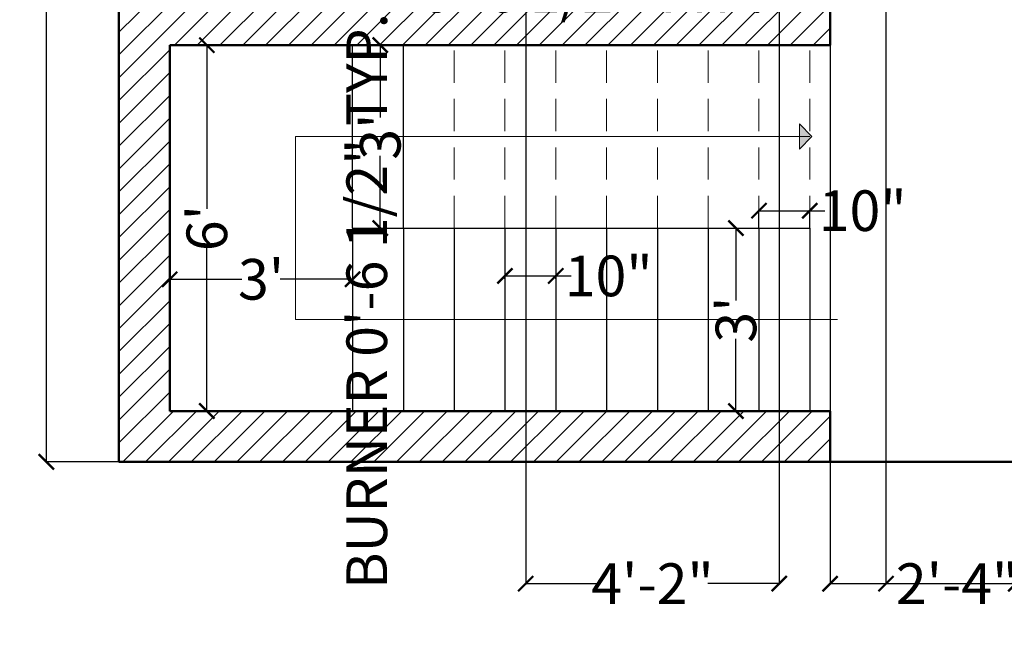
# Model space of a CAD drawing. Units: inches. Extents: x 1945 to 2401, y 1770 to 2289.
# Tile 1 of 5: x 1983 to 2177, y 1770 to 1893. Entities that reach past the tile are written whole.
import ezdxf

# ---------------------------------------------------------------- set-up
doc = ezdxf.new("R2010")
doc.units = ezdxf.units.IN
doc.linetypes.add('HIDDEN', pattern=[9.525, 6.35, -3.175])
for name, color, linetype, lineweight in [('A-ANNO-DIMS', 2, 'Continuous', 18), ('A-ANNO-SYMB', 50, 'Continuous', 18), ('A-FLOR-STRS-HIDN', 50, 'HIDDEN', 18), ('A-WALL-PATT', 8, 'Continuous', 13), ('Stairs', 50, 'Continuous', 25), ('Walls', 7, 'Continuous', 50)]:
    doc.layers.add(name, color=color, linetype=linetype, lineweight=lineweight)
doc.styles.get("Standard").update_dxf_attribs({"font": 'arial.ttf'})
doc.dimstyles.get("Standard").update_dxf_attribs({"dimtxt": 8, "dimasz": 3, "dimexe": 0.18, "dimexo": 0.0625, "dimgap": 0.09, "dimtad": 0, "dimdec": 1, "dimzin": 0, "dimdsep": 46, "dimlunit": 4, "dimtxsty": 'Standard', "dimblk": 'ARCHTICK', "dimcen": 0.09, "dimadec": 0, "dimazin": 0, "dimtfac": 1, "dimtdec": 1, "dimtofl": 0, "dimtmove": 0, "dimatfit": 3, "dimfxl": 1, "dimtolj": 1, "dimtzin": 0, "dimarcsym": 0})

# ---------------------------------------------------------------- blocks, each defined once
blk = doc.blocks.new('_ArchTick')
at = {"color": 0, "linetype": 'ByBlock', "const_width": 0.15}
blk.add_lwpolyline([(-0.5, -0.5), (0.5, 0.5)], dxfattribs=at)
blk = doc.blocks.new('*D13')
at = {"layer": 'A-ANNO-DIMS', "color": 0, "lineweight": -2, "transparency": 16777216}
for p, q in [((2123.03, 1852.04), (2124.49, 1852.04)), ((2124.31, 1852.04), (2124.31, 1837.81)), ((2124.31, 1816.04), (2124.31, 1830.27)), ((2123.03, 1816.04), (2124.49, 1816.04))]:
    blk.add_line(p, q, dxfattribs=at)
at = {"layer": 'Defpoints', "color": 0, "transparency": 16777216}
for p in [(2122.96, 1852.04), (2124.31, 1852.04), (2122.96, 1816.04)]:
    blk.add_point(p, dxfattribs=at)
at = {"layer": 'A-ANNO-DIMS', "color": 0, "lineweight": -2, "transparency": 16777216, "xscale": 3, "yscale": 3, "zscale": 3}
for p, rotation in [((2124.31, 1852.04), 90), ((2124.31, 1816.04), 270)]:
    blk.add_blockref('_ArchTick', p, dxfattribs=dict(at, rotation=rotation))
at = {"layer": 'A-ANNO-DIMS', "color": 0, "transparency": 16777216, "insert": (2124.31, 1834.04), "char_height": 8, "attachment_point": 5, "rotation": 90}
blk.add_mtext("\\A1;3'", dxfattribs=at)
blk = doc.blocks.new('*D14')
at = {"layer": 'A-ANNO-DIMS', "color": 0, "lineweight": -2, "transparency": 16777216}
for p, q in [((2048.9, 1888.04), (2054.47, 1888.04)), ((2054.29, 1888.04), (2054.29, 1873.81)), ((2054.29, 1852.04), (2054.29, 1866.27)), ((2048.9, 1852.04), (2054.47, 1852.04))]:
    blk.add_line(p, q, dxfattribs=at)
at = {"layer": 'Defpoints', "color": 0, "transparency": 16777216}
for p in [(2048.84, 1888.04), (2048.84, 1852.04), (2054.29, 1852.04)]:
    blk.add_point(p, dxfattribs=at)
at = {"layer": 'A-ANNO-DIMS', "color": 0, "lineweight": -2, "transparency": 16777216, "xscale": 3, "yscale": 3, "zscale": 3}
for p, rotation in [((2054.29, 1888.04), 90), ((2054.29, 1852.04), 270)]:
    blk.add_blockref('_ArchTick', p, dxfattribs=dict(at, rotation=rotation))
at = {"layer": 'A-ANNO-DIMS', "color": 0, "transparency": 16777216, "insert": (2054.29, 1870.04), "char_height": 8, "attachment_point": 5, "rotation": 90}
blk.add_mtext("\\A1;3'", dxfattribs=at)
blk = doc.blocks.new('*D15')
at = {"layer": 'A-ANNO-DIMS', "color": 0, "lineweight": -2, "transparency": 16777216}
for p, q in [((2012.9, 1888.04), (2020.33, 1888.04)), ((2020.15, 1888.04), (2020.15, 1855.83)), ((2020.15, 1816.04), (2020.15, 1848.25)), ((2012.9, 1816.04), (2020.33, 1816.04))]:
    blk.add_line(p, q, dxfattribs=at)
at = {"layer": 'Defpoints', "color": 0, "transparency": 16777216}
for p in [(2012.84, 1888.04), (2020.15, 1888.04), (2012.84, 1816.04)]:
    blk.add_point(p, dxfattribs=at)
at = {"layer": 'A-ANNO-DIMS', "color": 0, "lineweight": -2, "transparency": 16777216, "xscale": 3, "yscale": 3, "zscale": 3}
for p, rotation in [((2020.15, 1888.04), 90), ((2020.15, 1816.04), 270)]:
    blk.add_blockref('_ArchTick', p, dxfattribs=dict(at, rotation=rotation))
at = {"layer": 'A-ANNO-DIMS', "color": 0, "transparency": 16777216, "insert": (2020.15, 1852.04), "char_height": 8, "attachment_point": 5, "rotation": 90}
blk.add_mtext("\\A1;6'", dxfattribs=at)
blk = doc.blocks.new('*D16')
at = {"layer": 'A-ANNO-DIMS', "color": 0, "lineweight": -2, "transparency": 16777216}
for p, q in [((2012.84, 1851.98), (2012.84, 1841.78)), ((2048.84, 1851.98), (2048.84, 1841.78)), ((2012.84, 1841.96), (2027.07, 1841.96)), ((2048.84, 1841.96), (2034.61, 1841.96))]:
    blk.add_line(p, q, dxfattribs=at)
at = {"layer": 'Defpoints', "color": 0, "transparency": 16777216}
for p in [(2012.84, 1852.04), (2048.84, 1852.04), (2012.84, 1841.96)]:
    blk.add_point(p, dxfattribs=at)
at = {"layer": 'A-ANNO-DIMS', "color": 0, "lineweight": -2, "transparency": 16777216, "xscale": 3, "yscale": 3, "zscale": 3, "rotation": 180}
blk.add_blockref('_ArchTick', (2012.84, 1841.96), dxfattribs=at)
at = {"layer": 'A-ANNO-DIMS', "color": 0, "lineweight": -2, "transparency": 16777216, "xscale": 3, "yscale": 3, "zscale": 3}
blk.add_blockref('_ArchTick', (2048.84, 1841.96), dxfattribs=at)
at = {"layer": 'A-ANNO-DIMS', "color": 0, "transparency": 16777216, "insert": (2030.84, 1841.96), "char_height": 8, "attachment_point": 5}
blk.add_mtext("\\A1;3'", dxfattribs=at)
blk = doc.blocks.new('*D17')
at = {"layer": 'A-ANNO-DIMS', "color": 0, "lineweight": -2, "transparency": 16777216}
for p, q in [((2078.84, 1842.02), (2078.84, 1842.8)), ((2078.84, 1842.62), (2088.84, 1842.62)), ((2088.84, 1842.02), (2088.84, 1842.8)), ((2088.84, 1842.62), (2091.84, 1842.62))]:
    blk.add_line(p, q, dxfattribs=at)
at = {"layer": 'Defpoints', "color": 0, "transparency": 16777216}
for p in [(2078.84, 1841.96), (2088.84, 1842.62), (2088.84, 1841.96)]:
    blk.add_point(p, dxfattribs=at)
at = {"layer": 'A-ANNO-DIMS', "color": 0, "lineweight": -2, "transparency": 16777216, "xscale": 3, "yscale": 3, "zscale": 3, "rotation": 180}
blk.add_blockref('_ArchTick', (2078.84, 1842.62), dxfattribs=at)
at = {"layer": 'A-ANNO-DIMS', "color": 0, "lineweight": -2, "transparency": 16777216, "xscale": 3, "yscale": 3, "zscale": 3}
blk.add_blockref('_ArchTick', (2088.84, 1842.62), dxfattribs=at)
at = {"layer": 'A-ANNO-DIMS', "color": 0, "transparency": 16777216, "insert": (2099.26, 1842.62), "char_height": 8, "attachment_point": 5}
blk.add_mtext('\\A1;10"', dxfattribs=at)
blk = doc.blocks.new('*D18')
at = {"layer": 'A-ANNO-DIMS', "color": 0, "lineweight": -2, "transparency": 16777216}
for p, q in [((2128.84, 1852.1), (2128.84, 1855.64)), ((2128.84, 1855.46), (2138.84, 1855.46)), ((2138.84, 1852.1), (2138.84, 1855.64)), ((2138.84, 1855.46), (2141.84, 1855.46))]:
    blk.add_line(p, q, dxfattribs=at)
at = {"layer": 'Defpoints', "color": 0, "transparency": 16777216}
for p in [(2138.84, 1855.46), (2128.84, 1852.04), (2138.84, 1852.04)]:
    blk.add_point(p, dxfattribs=at)
at = {"layer": 'A-ANNO-DIMS', "color": 0, "lineweight": -2, "transparency": 16777216, "xscale": 3, "yscale": 3, "zscale": 3, "rotation": 180}
blk.add_blockref('_ArchTick', (2128.84, 1855.46), dxfattribs=at)
at = {"layer": 'A-ANNO-DIMS', "color": 0, "lineweight": -2, "transparency": 16777216, "xscale": 3, "yscale": 3, "zscale": 3}
blk.add_blockref('_ArchTick', (2138.84, 1855.46), dxfattribs=at)
at = {"layer": 'A-ANNO-DIMS', "color": 0, "transparency": 16777216, "insert": (2149.26, 1855.46), "char_height": 8, "attachment_point": 5}
blk.add_mtext('\\A1;10"', dxfattribs=at)
blk = doc.blocks.new('*D20')
at = {"layer": 'A-ANNO-DIMS', "color": 0, "lineweight": -2, "transparency": 16777216}
for p, q in [((2002.78, 2253.04), (1988.38, 2253.04)), ((1988.56, 2253.04), (1988.56, 2043.37)), ((1988.56, 1806.04), (1988.56, 2015.71)), ((2002.78, 1806.04), (1988.38, 1806.04))]:
    blk.add_line(p, q, dxfattribs=at)
at = {"layer": 'Defpoints', "color": 0, "transparency": 16777216}
for p in [(2002.84, 2253.04), (1988.56, 1806.04), (2002.84, 1806.04)]:
    blk.add_point(p, dxfattribs=at)
at = {"layer": 'A-ANNO-DIMS', "color": 0, "lineweight": -2, "transparency": 16777216, "xscale": 3, "yscale": 3, "zscale": 3}
for p, rotation in [((1988.56, 2253.04), 90), ((1988.56, 1806.04), 270)]:
    blk.add_blockref('_ArchTick', p, dxfattribs=dict(at, rotation=rotation))
at = {"layer": 'A-ANNO-DIMS', "color": 0, "transparency": 16777216, "insert": (1988.56, 2029.54), "char_height": 8, "attachment_point": 5, "rotation": 90}
blk.add_mtext('\\A1;37\'-3"', dxfattribs=at)
blk = doc.blocks.new('*D29')
at = {"layer": 'A-ANNO-DIMS', "color": 0, "lineweight": -2, "transparency": 16777216}
for p, q in [((2052.57, 1906.21), (2051.45, 1906.21)), ((2051.63, 1906.21), (2051.63, 1899.48)), ((2052.57, 1899.48), (2051.45, 1899.48)), ((2051.63, 1899.48), (2051.63, 1896.48))]:
    blk.add_line(p, q, dxfattribs=at)
at = {"layer": 'Defpoints', "color": 0, "transparency": 16777216}
for p in [(2052.64, 1906.21), (2051.63, 1899.48), (2052.64, 1899.48)]:
    blk.add_point(p, dxfattribs=at)
at = {"layer": 'A-ANNO-DIMS', "color": 0, "lineweight": -2, "transparency": 16777216, "xscale": 3, "yscale": 3, "zscale": 3}
for p, rotation in [((2051.63, 1906.21), 90), ((2051.63, 1899.48), 270)]:
    blk.add_blockref('_ArchTick', p, dxfattribs=dict(at, rotation=rotation))
at = {"layer": 'A-ANNO-DIMS', "color": 0, "transparency": 16777216, "insert": (2051.63, 1837.71), "char_height": 8, "attachment_point": 5, "rotation": 90}
blk.add_mtext('\\A1;BURNER 0\'-6 1/2" TYP.', dxfattribs=at)
blk = doc.blocks.new('*D30')
at = {"layer": 'A-ANNO-DIMS', "color": 0, "lineweight": -2, "transparency": 16777216}
for p, q in [((2052.64, 1899.41), (2052.64, 1898.29)), ((2052.64, 1898.47), (2059.37, 1898.47)), ((2059.37, 1899.41), (2059.37, 1898.29)), ((2059.37, 1898.47), (2062.37, 1898.47))]:
    blk.add_line(p, q, dxfattribs=at)
at = {"layer": 'Defpoints', "color": 0, "transparency": 16777216}
for p in [(2052.64, 1899.48), (2059.37, 1899.48), (2059.37, 1898.47)]:
    blk.add_point(p, dxfattribs=at)
at = {"layer": 'A-ANNO-DIMS', "color": 0, "lineweight": -2, "transparency": 16777216, "xscale": 3, "yscale": 3, "zscale": 3, "rotation": 180}
blk.add_blockref('_ArchTick', (2052.64, 1898.47), dxfattribs=at)
at = {"layer": 'A-ANNO-DIMS', "color": 0, "lineweight": -2, "transparency": 16777216, "xscale": 3, "yscale": 3, "zscale": 3}
blk.add_blockref('_ArchTick', (2059.37, 1898.47), dxfattribs=at)
at = {"layer": 'A-ANNO-DIMS', "color": 0, "transparency": 16777216, "insert": (2096.16, 1898.47), "char_height": 8, "attachment_point": 5}
blk.add_mtext('\\A1;0\'-6 1/2" TYP.', dxfattribs=at)
blk = doc.blocks.new('*D65')
at = {"layer": 'A-ANNO-DIMS', "color": 0, "lineweight": -2, "transparency": 16777216}
for p, q in [((2142.84, 1910.98), (2142.84, 1781.89)), ((2179.42, 1910.98), (2179.42, 1781.89)), ((2142.84, 1782.07), (2179.42, 1782.07)), ((2179.42, 1782.07), (2182.42, 1782.07))]:
    blk.add_line(p, q, dxfattribs=at)
at = {"layer": 'Defpoints', "color": 0, "transparency": 16777216}
for p in [(2142.84, 1911.04), (2179.42, 1911.04), (2179.42, 1782.07)]:
    blk.add_point(p, dxfattribs=at)
at = {"layer": 'A-ANNO-DIMS', "color": 0, "lineweight": -2, "transparency": 16777216, "xscale": 3, "yscale": 3, "zscale": 3, "rotation": 180}
blk.add_blockref('_ArchTick', (2142.84, 1782.07), dxfattribs=at)
at = {"layer": 'A-ANNO-DIMS', "color": 0, "lineweight": -2, "transparency": 16777216, "xscale": 3, "yscale": 3, "zscale": 3}
blk.add_blockref('_ArchTick', (2179.42, 1782.07), dxfattribs=at)
at = {"layer": 'A-ANNO-DIMS', "color": 0, "transparency": 16777216, "insert": (2202.46, 1782.07), "char_height": 8, "attachment_point": 5}
blk.add_mtext('\\A1;3\'-0 1/2"', dxfattribs=at)
blk = doc.blocks.new('*D69')
at = {"layer": 'A-ANNO-DIMS', "color": 0, "lineweight": -2, "transparency": 16777216}
for p, q in [((2132.84, 2005.98), (2132.84, 1781.89)), ((2082.92, 1999.98), (2082.92, 1781.89)), ((2082.92, 1782.07), (2097, 1782.07)), ((2132.84, 1782.07), (2118.77, 1782.07))]:
    blk.add_line(p, q, dxfattribs=at)
at = {"layer": 'Defpoints', "color": 0, "transparency": 16777216}
for p in [(2132.84, 2006.04), (2082.92, 2000.04), (2132.84, 1782.07)]:
    blk.add_point(p, dxfattribs=at)
at = {"layer": 'A-ANNO-DIMS', "color": 0, "lineweight": -2, "transparency": 16777216, "xscale": 3, "yscale": 3, "zscale": 3, "rotation": 180}
blk.add_blockref('_ArchTick', (2082.92, 1782.07), dxfattribs=at)
at = {"layer": 'A-ANNO-DIMS', "color": 0, "lineweight": -2, "transparency": 16777216, "xscale": 3, "yscale": 3, "zscale": 3}
blk.add_blockref('_ArchTick', (2132.84, 1782.07), dxfattribs=at)
at = {"layer": 'A-ANNO-DIMS', "color": 0, "transparency": 16777216, "insert": (2107.88, 1782.07), "char_height": 8, "attachment_point": 5}
blk.add_mtext('\\A1;4\'-2"', dxfattribs=at)
blk = doc.blocks.new('*D70')
at = {"layer": 'A-ANNO-DIMS', "color": 0, "lineweight": -2, "transparency": 16777216}
for p, q in [((2153.84, 2100.98), (2153.84, 1781.89)), ((2181.84, 2100.98), (2181.84, 1781.89)), ((2153.84, 1782.07), (2157.05, 1782.07)), ((2181.84, 1782.07), (2178.63, 1782.07))]:
    blk.add_line(p, q, dxfattribs=at)
at = {"layer": 'Defpoints', "color": 0, "transparency": 16777216}
for p in [(2153.84, 2101.04), (2181.84, 2101.04), (2181.84, 1782.07)]:
    blk.add_point(p, dxfattribs=at)
at = {"layer": 'A-ANNO-DIMS', "color": 0, "lineweight": -2, "transparency": 16777216, "xscale": 3, "yscale": 3, "zscale": 3, "rotation": 180}
blk.add_blockref('_ArchTick', (2153.84, 1782.07), dxfattribs=at)
at = {"layer": 'A-ANNO-DIMS', "color": 0, "lineweight": -2, "transparency": 16777216, "xscale": 3, "yscale": 3, "zscale": 3}
blk.add_blockref('_ArchTick', (2181.84, 1782.07), dxfattribs=at)
at = {"layer": 'A-ANNO-DIMS', "color": 0, "transparency": 16777216, "insert": (2167.84, 1782.07), "char_height": 8, "attachment_point": 5}
blk.add_mtext('\\A1;2\'-4"', dxfattribs=at)

msp = doc.modelspace()

# ---------------------------------------------------------------- hatches: boundary and pattern name
at = {"layer": 'A-ANNO-SYMB'}
h = msp.add_hatch(color=256, dxfattribs=at)
h.dxf.hatch_style = 1
h.paths.add_polyline_path([(2136.79, 1867.57), (2139.26, 1870.04), (2136.79, 1872.52)])
at = {"layer": 'A-WALL-PATT', "transparency": 33554585}
h = msp.add_hatch(dxfattribs=at)
h.set_pattern_fill('ANSI31', color=256)
h.paths.add_polyline_path([(2142.84, 2006.04), (2132.84, 2006.04), (2132.84, 1898.04), (2012.84, 1898.04), (2012.84, 1888.04), (2142.84, 1888.04), (2142.84, 1911.04), (2179.42, 1911.04), (2179.42, 1921.04), (2142.84, 1921.04)])
h.paths.add_polyline_path([(2269.5, 1921.04), (2239.42, 1921.04), (2239.42, 1911.04), (2269.5, 1911.04)])
h.paths.add_polyline_path([(2332.84, 1981.04), (2322.84, 1981.04), (2322.84, 1921.04), (2311.84, 1921.04), (2311.84, 1911.04), (2322.84, 1911.04), (2322.84, 1817.97), (2332.84, 1817.97)])
h.paths.add_polyline_path([(2012.84, 1931.04), (2002.84, 1931.04), (2002.84, 1806.04), (2142.84, 1806.04), (2142.84, 1816.04), (2012.84, 1816.04)])
h.paths.add_polyline_path([(2012.84, 2000.04), (2082.92, 2000.04), (2082.92, 2006.04), (2066.84, 2006.04), (2066.84, 2101.04), (2142.84, 2101.04), (2153.84, 2101.04), (2153.84, 2111.04), (2142.84, 2111.04), (2142.84, 2118.04), (2132.84, 2118.04), (2132.84, 2111.04), (2060.84, 2111.04), (2060.84, 2006.04), (2012.84, 2006.04), (2012.84, 2026.45), (2002.84, 2026.45), (2002.84, 1967.04), (2012.84, 1967.04)])

# ---------------------------------------------------------------- linework, layer by layer
at = {"layer": 'A-ANNO-SYMB'}
for p, q in [((2136.79, 1872.52), (2136.79, 1867.57)), ((2139.26, 1870.04), (2136.79, 1872.52)), ((2037.59, 1834.04), (2037.59, 1870.04)), ((2037.59, 1870.04), (2138.84, 1870.04)), ((2139.26, 1870.04), (2136.79, 1867.57)), ((2144.33, 1834.04), (2037.59, 1834.04))]:
    msp.add_line(p, q, dxfattribs=at)
at = {"layer": 'A-FLOR-STRS-HIDN'}
for p, q in [((2068.84, 1852.04), (2068.84, 1888.04)), ((2078.84, 1852.04), (2078.84, 1888.04)), ((2088.84, 1852.04), (2088.84, 1888.04)), ((2098.84, 1852.04), (2098.84, 1888.04)), ((2108.84, 1852.04), (2108.84, 1888.04)), ((2118.84, 1852.04), (2118.84, 1888.04)), ((2128.84, 1852.04), (2128.84, 1888.04)), ((2138.84, 1852.04), (2138.84, 1888.04))]:
    msp.add_line(p, q, dxfattribs=at)
at = {"layer": 'Stairs'}
for p, q in [((2048.84, 1852.04), (2048.84, 1888.04)), ((2058.84, 1852.04), (2058.84, 1888.04)), ((2048.84, 1852.04), (2048.84, 1816.04)), ((2048.84, 1852.04), (2138.84, 1852.04)), ((2058.84, 1852.04), (2058.84, 1816.04)), ((2068.84, 1852.04), (2068.84, 1816.04)), ((2078.84, 1852.04), (2078.84, 1816.04)), ((2088.84, 1852.04), (2088.84, 1816.04)), ((2098.84, 1852.04), (2098.84, 1816.04)), ((2108.84, 1852.04), (2108.84, 1816.04)), ((2118.84, 1852.04), (2118.84, 1816.04)), ((2128.84, 1852.04), (2128.84, 1816.04)), ((2138.84, 1852.04), (2138.84, 1816.04))]:
    msp.add_line(p, q, dxfattribs=at)
at = {"layer": 'Walls'}
for p, q in [((2002.84, 2253.04), (2002.84, 1806.04)), ((2142.84, 1911.04), (2142.84, 1888.04)), ((2012.84, 1888.04), (2142.84, 1888.04)), ((2012.84, 1888.04), (2012.84, 1816.04)), ((2012.84, 1816.04), (2142.84, 1816.04)), ((2142.84, 1816.04), (2142.84, 1806.04)), ((2002.84, 1806.04), (2322.84, 1806.04))]:
    msp.add_line(p, q, dxfattribs=at)

# ---------------------------------------------------------------- dimensions: what is measured, and where the dimension line sits
at = {"layer": 'A-ANNO-DIMS'}
for base, p1, p2, picture, middle in [((1988.56, 1806.04), (2002.84, 2253.04), (2002.84, 1806.04), '*D20', (1988.56, 2029.54)), ((2020.15, 1888.04), (2012.84, 1816.04), (2012.84, 1888.04), '*D15', (2020.15, 1852.04)), ((2054.29, 1852.04), (2048.84, 1888.04), (2048.84, 1852.04), '*D14', (2054.29, 1870.04)), ((2124.31, 1852.04), (2122.96, 1816.04), (2122.96, 1852.04), '*D13', (2124.31, 1834.04))]:
    dim = msp.add_linear_dim(base=base, p1=p1, p2=p2, angle=90, dimstyle='Standard', override={"dimclrd": 0, "dimclre": 0, "dimclrt": 0}, dxfattribs=at)
    dim.commit()
    dim.dimension.update_dxf_attribs({"geometry": picture, "text_midpoint": middle})
for base, p1, p2, override, picture, middle in [((2181.84, 1782.07), (2153.84, 2101.04), (2181.84, 2101.04), {"dimdec": 1, "dimlfac": 1, "dimrnd": 0, "dimzin": 1, "dimdsep": 46, "dimlunit": 4, "dimfrac": 2}, '*D70', (2167.84, 1782.07)), ((2132.84, 1782.07), (2082.92, 2000.04), (2132.84, 2006.04), {"dimdec": 1, "dimlfac": 1, "dimrnd": 0, "dimzin": 1, "dimdsep": 46, "dimlunit": 4, "dimfrac": 2}, '*D69', (2107.88, 1782.07)), ((2179.42, 1782.07), (2142.84, 1911.04), (2179.42, 1911.04), {"dimdec": 1, "dimlfac": 1, "dimrnd": 0, "dimzin": 1, "dimdsep": 46, "dimlunit": 4, "dimfrac": 2}, '*D65', (2202.46, 1782.07)), ((2138.84, 1855.46), (2128.84, 1852.04), (2138.84, 1852.04), {"dimclrd": 0, "dimclre": 0, "dimclrt": 0}, '*D18', (2149.26, 1855.46)), ((2012.84, 1841.96), (2048.84, 1852.04), (2012.84, 1852.04), {"dimclrd": 0, "dimclre": 0, "dimclrt": 0}, '*D16', (2030.84, 1841.96)), ((2088.84, 1842.62), (2078.84, 1841.96), (2088.84, 1841.96), {"dimclrd": 0, "dimclre": 0, "dimclrt": 0}, '*D17', (2099.26, 1842.62))]:
    dim = msp.add_linear_dim(base=base, p1=p1, p2=p2, dimstyle='Standard', override=override, dxfattribs=at)
    dim.commit()
    dim.dimension.update_dxf_attribs({"geometry": picture, "text_midpoint": middle})
dim = msp.add_linear_dim(base=(2059.37, 1898.47), p1=(2052.64, 1899.48), p2=(2059.37, 1899.48), text='<> TYP.', dimstyle='Standard', override={"dimdec": 1, "dimlfac": 1, "dimrnd": 0, "dimzin": 1, "dimdsep": 46, "dimlunit": 4, "dimfrac": 2}, dxfattribs=at)
dim.commit()
dim.dimension.update_dxf_attribs({"geometry": '*D30', "text_midpoint": (2096.16, 1898.47)})
dim = msp.add_linear_dim(base=(2051.63, 1899.48), p1=(2052.64, 1906.21), p2=(2052.64, 1899.48), angle=270, text='BURNER <> TYP.', dimstyle='Standard', override={"dimdec": 1, "dimlfac": 1, "dimrnd": 0, "dimzin": 1, "dimdsep": 46, "dimlunit": 4, "dimfrac": 2}, dxfattribs=at)
dim.commit()
dim.dimension.update_dxf_attribs({"geometry": '*D29', "text_midpoint": (2051.63, 1837.71)})

doc.saveas('drawing.dxf')
